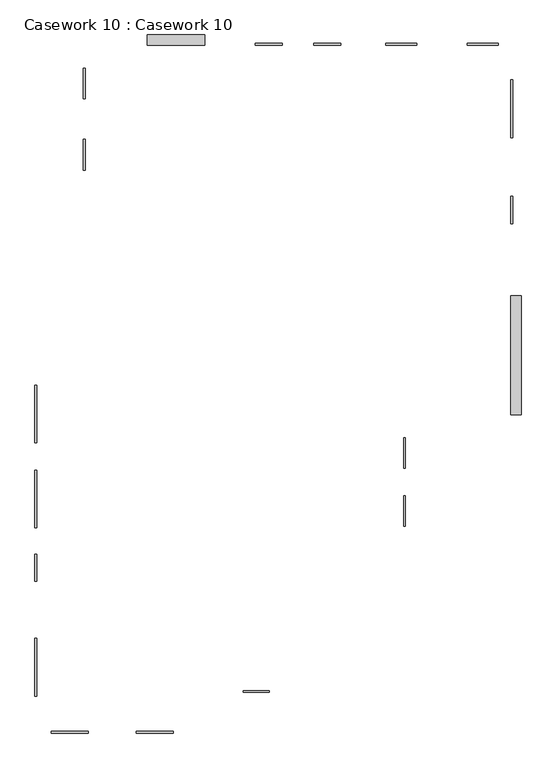
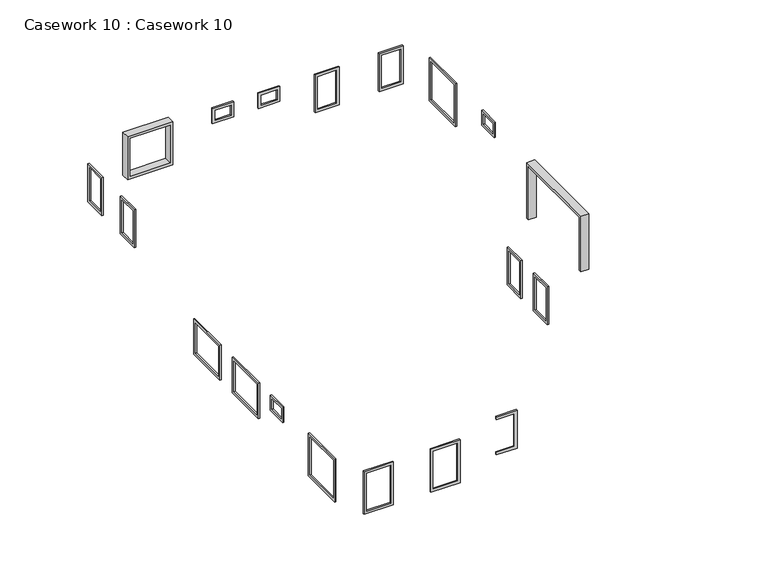
"""IFC4 building model written with IfcOpenShell, lengths in millimetres: furniture geometry, Casework 10 : Casework 10."""

from ifc_helpers import new_model, si_unit, frame, origin, place, context, project, spatial, polyline, outline, extrude, source, transform, mapped, element, save


def casework_10_casework_10_bcdbd455(model_context):
    return source(origin(), model_context, "Body", "SweptSolid", [
        extrude(outline(polyline([(1615.8070837, 2550.0), (-1684.1929163, 2550.0), (-1684.1929163, 450.0), (-1784.1929163, 450.0), (-1784.1929163, 2650.0), (1715.8070837, 2650.0), (1715.8070837, 450.0), (1615.8070837, 450.0), (1615.8070837, 2550.0)])), frame((7838.2046034, 0.0, 0.0), z_axis=(1.0, 0.0, 0.0), x_axis=(0.0, 1.0, 0.0)), (0.0, 0.0, 1.0), 300.0),
        extrude(outline(polyline([(-4159.1929163, 2940.0), (-4159.1929163, 1440.0), (-5059.1929163, 1440.0), (-5059.1929163, 2940.0), (-4159.1929163, 2940.0)]), holes=[polyline([(-4259.1929163, 2840.0), (-4959.1929163, 2840.0), (-4959.1929163, 1540.0), (-4259.1929163, 1540.0), (-4259.1929163, 2840.0)])]), frame((4688.2046034, 0.0, 0.0), z_axis=(1.0, 0.0, 0.0), x_axis=(0.0, 1.0, 0.0)), (0.0, 0.0, 1.0), 50.0),
        extrude(outline(polyline([(-2459.1929163, 2940.0), (-2459.1929163, 1440.0), (-3359.1929163, 1440.0), (-3359.1929163, 2940.0), (-2459.1929163, 2940.0)]), holes=[polyline([(-2559.1929163, 2840.0), (-3259.1929163, 2840.0), (-3259.1929163, 1540.0), (-2559.1929163, 1540.0), (-2559.1929163, 2840.0)])]), frame((4688.2046034, 0.0, 0.0), z_axis=(1.0, 0.0, 0.0), x_axis=(0.0, 1.0, 0.0)), (0.0, 0.0, 1.0), 50.0),
        extrude(outline(polyline([(4640.8070837, 2950.0), (4640.8070837, 2350.0), (3840.8070837, 2350.0), (3840.8070837, 2950.0), (4640.8070837, 2950.0)]), holes=[polyline([(4540.8070837, 2850.0), (3940.8070837, 2850.0), (3940.8070837, 2450.0), (4540.8070837, 2450.0), (4540.8070837, 2850.0)])]), frame((7838.2046034, 0.0, 0.0), z_axis=(1.0, 0.0, 0.0), x_axis=(0.0, 1.0, 0.0)), (0.0, 0.0, 1.0), 50.0),
        extrude(outline(polyline([(8065.8070837, 2950.0), (8065.8070837, 1250.0), (6365.8070837, 1250.0), (6365.8070837, 2950.0), (8065.8070837, 2950.0)]), holes=[polyline([(7965.8070837, 2850.0), (6465.8070837, 2850.0), (6465.8070837, 1350.0), (7965.8070837, 1350.0), (7965.8070837, 2850.0)])]), frame((7838.2046034, 0.0, 0.0), z_axis=(1.0, 0.0, 0.0), x_axis=(0.0, 1.0, 0.0)), (0.0, 0.0, 1.0), 50.0),
        extrude(outline(polyline([(2950.0, 2838.2046034), (2950.0, 2038.2046034), (2350.0, 2038.2046034), (2350.0, 2838.2046034), (2950.0, 2838.2046034)]), holes=[polyline([(2850.0, 2138.2046034), (2850.0, 2738.2046034), (2450.0, 2738.2046034), (2450.0, 2138.2046034), (2850.0, 2138.2046034)])]), frame((0.0, 9090.8070837, 0.0), z_axis=(0.0, 1.0, 0.0), x_axis=(0.0, 0.0, 1.0)), (0.0, 0.0, 1.0), 50.0),
        extrude(outline(polyline([(2950.0, 1113.2046034), (2950.0, 313.2046034), (2350.0, 313.2046034), (2350.0, 1113.2046034), (2950.0, 1113.2046034)]), holes=[polyline([(2850.0, 413.2046034), (2850.0, 1013.2046034), (2450.0, 1013.2046034), (2450.0, 413.2046034), (2850.0, 413.2046034)])]), frame((0.0, 9090.8070837, 0.0), z_axis=(0.0, 1.0, 0.0), x_axis=(0.0, 0.0, 1.0)), (0.0, 0.0, 1.0), 50.0),
        extrude(outline(polyline([(2940.0, 6563.2046034), (1440.0, 6563.2046034), (1440.0, 7463.2046034), (2940.0, 7463.2046034), (2940.0, 6563.2046034)]), holes=[polyline([(2840.0, 6663.2046034), (2840.0, 7363.2046034), (1540.0, 7363.2046034), (1540.0, 6663.2046034), (2840.0, 6663.2046034)])]), frame((0.0, 9090.8070837, 0.0), z_axis=(0.0, 1.0, 0.0), x_axis=(0.0, 0.0, 1.0)), (0.0, 0.0, 1.0), 50.0),
        extrude(outline(polyline([(2940.0, 5063.2046034), (2940.0, 4163.2046034), (1440.0, 4163.2046034), (1440.0, 5063.2046034), (2940.0, 5063.2046034)]), holes=[polyline([(1540.0, 4263.2046034), (2840.0, 4263.2046034), (2840.0, 4963.2046034), (1540.0, 4963.2046034), (1540.0, 4263.2046034)])]), frame((0.0, 9090.8070837, 0.0), z_axis=(0.0, 1.0, 0.0), x_axis=(0.0, 0.0, 1.0)), (0.0, 0.0, 1.0), 50.0),
        extrude(outline(polyline([(2950.0, -2861.7953966), (1250.0, -2861.7953966), (1250.0, -1161.7953966), (2950.0, -1161.7953966), (2950.0, -2861.7953966)]), holes=[polyline([(2850.0, -2761.7953966), (2850.0, -1261.7953966), (1350.0, -1261.7953966), (1350.0, -2761.7953966), (2850.0, -2761.7953966)])]), frame((0.0, 9090.8070837, 0.0), z_axis=(0.0, 1.0, 0.0), x_axis=(0.0, 0.0, 1.0)), (0.0, 0.0, 1.0), 300.0),
        extrude(outline(polyline([(7515.8070837, 2940.0), (8415.8070837, 2940.0), (8415.8070837, 1440.0), (7515.8070837, 1440.0), (7515.8070837, 2940.0)]), holes=[polyline([(7615.8070837, 2840.0), (7615.8070837, 1540.0), (8315.8070837, 1540.0), (8315.8070837, 2840.0), (7615.8070837, 2840.0)])]), frame((-4736.7953966, 0.0, 0.0), z_axis=(1.0, 0.0, 0.0), x_axis=(0.0, 1.0, 0.0)), (0.0, 0.0, 1.0), 50.0),
        extrude(outline(polyline([(5415.8070837, 2940.0), (6315.8070837, 2940.0), (6315.8070837, 1440.0), (5415.8070837, 1440.0), (5415.8070837, 2940.0)]), holes=[polyline([(5515.8070837, 2840.0), (5515.8070837, 1540.0), (6215.8070837, 1540.0), (6215.8070837, 2840.0), (5515.8070837, 2840.0)])]), frame((-4736.7953966, 0.0, 0.0), z_axis=(1.0, 0.0, 0.0), x_axis=(0.0, 1.0, 0.0)), (0.0, 0.0, 1.0), 50.0),
        extrude(outline(polyline([(-10059.1929163, 2950.0), (-8359.1929163, 2950.0), (-8359.1929163, 1250.0), (-10059.1929163, 1250.0), (-10059.1929163, 2950.0)]), holes=[polyline([(-9959.1929163, 2850.0), (-9959.1929163, 1350.0), (-8459.1929163, 1350.0), (-8459.1929163, 2850.0), (-9959.1929163, 2850.0)])]), frame((-6161.7953966, 0.0, 0.0), z_axis=(1.0, 0.0, 0.0), x_axis=(0.0, 1.0, 0.0)), (0.0, 0.0, 1.0), 50.0),
        extrude(outline(polyline([(-2609.1929163, 2950.0), (-909.1929163, 2950.0), (-909.1929163, 1550.0), (-2609.1929163, 1550.0), (-2609.1929163, 2950.0)]), holes=[polyline([(-2509.1929163, 2850.0), (-2509.1929163, 1650.0), (-1009.1929163, 1650.0), (-1009.1929163, 2850.0), (-2509.1929163, 2850.0)])]), frame((-6161.7953966, 0.0, 0.0), z_axis=(1.0, 0.0, 0.0), x_axis=(0.0, 1.0, 0.0)), (0.0, 0.0, 1.0), 50.0),
        extrude(outline(polyline([(-5109.1929163, 2950.0), (-3409.1929163, 2950.0), (-3409.1929163, 1550.0), (-5109.1929163, 1550.0), (-5109.1929163, 2950.0)]), holes=[polyline([(-5009.1929163, 2850.0), (-5009.1929163, 1650.0), (-3509.1929163, 1650.0), (-3509.1929163, 2850.0), (-5009.1929163, 2850.0)])]), frame((-6161.7953966, 0.0, 0.0), z_axis=(1.0, 0.0, 0.0), x_axis=(0.0, 1.0, 0.0)), (0.0, 0.0, 1.0), 50.0),
        extrude(outline(polyline([(-6684.1929163, 2950.0), (-5884.1929163, 2950.0), (-5884.1929163, 2350.0), (-6684.1929163, 2350.0), (-6684.1929163, 2950.0)]), holes=[polyline([(-6584.1929163, 2850.0), (-6584.1929163, 2450.0), (-5984.1929163, 2450.0), (-5984.1929163, 2850.0), (-6584.1929163, 2850.0)])]), frame((-6161.7953966, 0.0, 0.0), z_axis=(1.0, 0.0, 0.0), x_axis=(0.0, 1.0, 0.0)), (0.0, 0.0, 1.0), 50.0),
        extrude(outline(polyline([(2300.0, 638.2046034), (1000.0, 638.2046034), (1000.0, -36.7953966), (900.0, -36.7953966), (900.0, 738.2046034), (2400.0, 738.2046034), (2400.0, -36.7953966), (2300.0, -36.7953966), (2300.0, 638.2046034)])), frame((0.0, -9946.6929163, 0.0), z_axis=(0.0, 1.0, 0.0), x_axis=(0.0, 0.0, 1.0)), (0.0, 0.0, 1.0), 50.0),
        extrude(outline(polyline([(2950.0, -3186.7953966), (1250.0, -3186.7953966), (1250.0, -2086.7953966), (2950.0, -2086.7953966), (2950.0, -3186.7953966)]), holes=[polyline([(2850.0, -2186.7953966), (1350.0, -2186.7953966), (1350.0, -3086.7953966), (2850.0, -3086.7953966), (2850.0, -2186.7953966)])]), frame((0.0, -11146.6929163, 0.0), z_axis=(0.0, 1.0, 0.0), x_axis=(0.0, 0.0, 1.0)), (0.0, 0.0, 1.0), 50.0),
        extrude(outline(polyline([(2950.0, -4586.7953966), (2950.0, -5686.7953966), (1250.0, -5686.7953966), (1250.0, -4586.7953966), (2950.0, -4586.7953966)]), holes=[polyline([(2850.0, -4686.7953966), (1350.0, -4686.7953966), (1350.0, -5586.7953966), (2850.0, -5586.7953966), (2850.0, -4686.7953966)])]), frame((0.0, -11146.6929163, 0.0), z_axis=(0.0, 1.0, 0.0), x_axis=(0.0, 0.0, 1.0)), (0.0, 0.0, 1.0), 50.0),
    ])


if __name__ == "__main__":
    model = new_model("IFC4")
    model_context = context("Model", 3, world=origin())
    ifc_project = project(units=[si_unit("LENGTHUNIT", "METRE", prefix="MILLI")], contexts=[model_context])
    site = spatial("IfcSite", under=ifc_project)
    building = spatial("IfcBuilding", under=site)
    placement = place(None, origin())
    casework_10_casework_10_shape = casework_10_casework_10_bcdbd455(model_context)
    element("IfcFurniture", 1, ObjectType="Casework 10 : Casework 10", at=placement, inside=building, context=model_context, shape_type="MappedRepresentation", body=[
        mapped(casework_10_casework_10_shape, transform((0.0, 0.0, 0.0), x_axis=(1.0, 0.0, 0.0), y_axis=(0.0, 1.0, 0.0), z_axis=(0.0, 0.0, 1.0))),
    ])
    save(model, "model.ifc")
